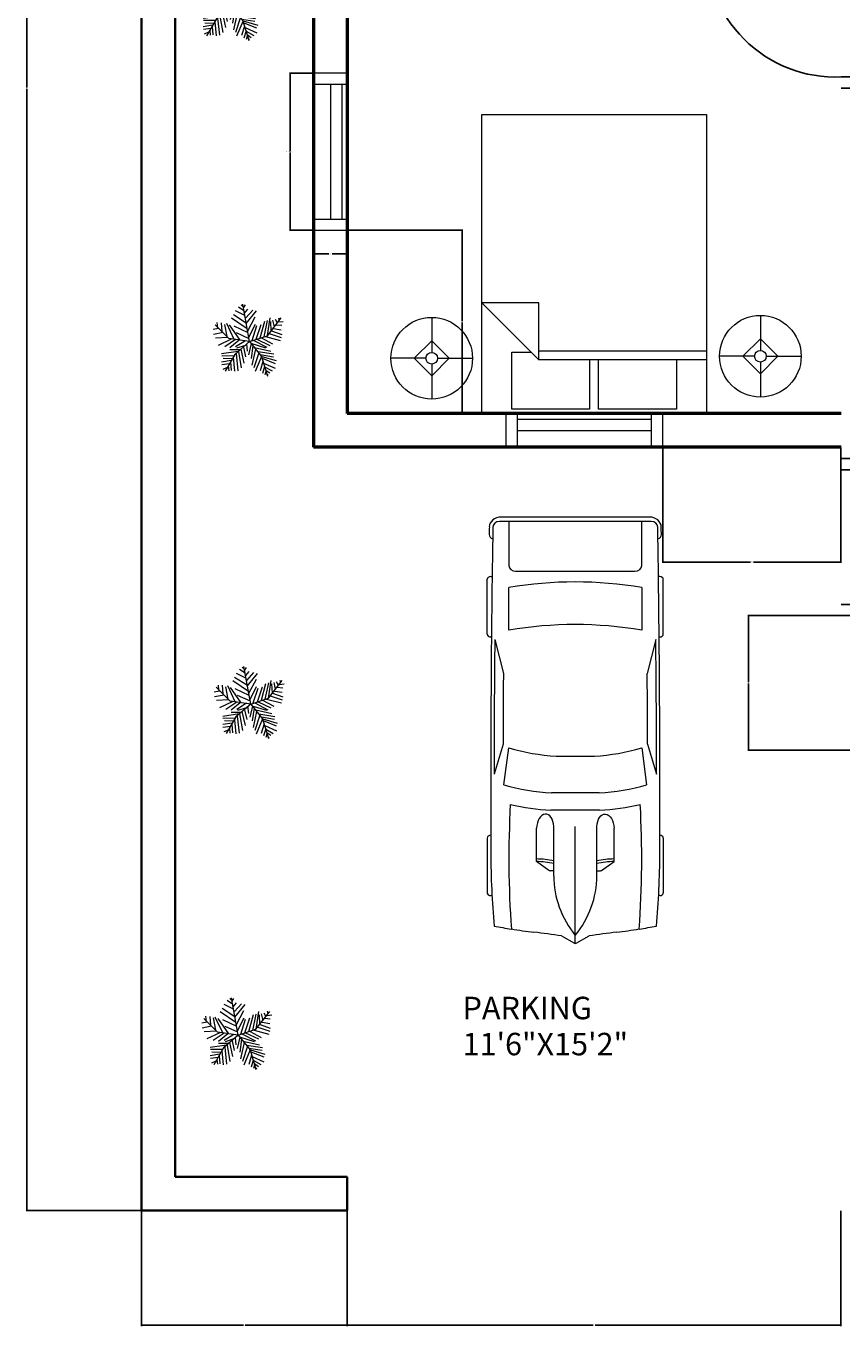
# Model space of a CAD drawing. Units: inches. Extents: x 156 to 720, y 11 to 679.
# Tile 1 of 5: x 156 to 374, y 11 to 359. Entities that reach past the tile are written whole.
import ezdxf

# ---------------------------------------------------------------- set-up
doc = ezdxf.new("R2010")
doc.units = ezdxf.units.IN
for name, color, linetype, lineweight in [('A-ANNO-DIMS', 2, 'Continuous', 18), ('A-AREA-IDEN', 7, 'Continuous', 25), ('A-DOOR', 3, 'Continuous', 25), ('A-FURN', 8, 'Continuous', 18), ('A-GLAZ', 4, 'Continuous', 18), ('A-WALL', 7, 'Continuous', 50), ('C-PKNG-VEHC', 8, 'Continuous', 13), ('C-PROP', 7, 'Continuous', 35), ('E-LITE', 2, 'Continuous', 13), ('L-PLNT', 94, 'Continuous', 13)]:
    doc.layers.add(name, color=color, linetype=linetype, lineweight=lineweight)
doc.styles.get("Standard").update_dxf_attribs({"font": 'arial.ttf'})
doc.dimstyles.get("Standard").update_dxf_attribs({"dimtxt": 0.18, "dimasz": 0.18, "dimexe": 0.18, "dimexo": 0.0625, "dimgap": 0.09, "dimtad": 0, "dimtih": 1, "dimtoh": 1, "dimdec": 4, "dimzin": 0, "dimdsep": 46, "dimtxsty": 'Standard', "dimcen": 0.09, "dimadec": 0, "dimazin": 0, "dimtfac": 1, "dimtdec": 4, "dimtofl": 0, "dimtmove": 0, "dimatfit": 3, "dimfxl": 1, "dimtolj": 1, "dimtzin": 0, "dimarcsym": 0})

# ---------------------------------------------------------------- blocks, each defined once
blk = doc.blocks.new('Bed - Queen')
for p, q in [((0, -80.00003), (0, 0)), ((0, 0), (59.99999, 0)), ((59.99999, 0), (59.99999, -80.00003)), ((7.99999, -1.2), (28.79998, -1.2)), ((7.99999, -14.4), (7.99999, -1.2)), ((28.79998, -1.2), (28.79998, -14.4)), ((31.19999, -1.2), (51.99999, -1.2)), ((31.19999, -14.4), (31.19999, -1.2)), ((51.99999, -1.2), (51.99999, -16.4)), ((0, -14.4), (44.8, -14.4)), ((44.8, -16.8), (0, -16.8)), ((59.99999, -29.6), (44.8, -14.4)), ((44.8, -14.4), (44.8, -29.6)), ((51.99999, -16.4), (46.79936, -16.4)), ((44.8, -29.6), (59.99999, -29.6)), ((59.99999, -80.00003), (0, -80.00003))]:
    blk.add_line(p, q)
blk = doc.blocks.new('Lamp - Table')
for p, q in [((0, 7), (0, 1)), ((0, 3), (-3, 0)), ((3, 0), (0, 3)), ((-1, 0), (-7, 0)), ((-3, 0), (0, -3)), ((0, -3), (3, 0)), ((1, 0), (7, 0)), ((0, -1), (0, -7))]:
    blk.add_line(p, q)
for radius in [7, 1]:
    blk.add_circle((0, 0), radius)
blk = doc.blocks.new('*U14')
for p, q in [((21.1, 37.41), (21.1, 36.83)), ((46.55, 38.89), (22.35, 38.89)), ((47.8, 37.39), (47.8, 37.41)), ((87.99, 31.87), (74.76, 35.92)), ((134.31, 35.6), (119.29, 31.78)), ((135.45, 37.07), (135.45, 37.41)), ((136.7, 38.89), (160.9, 38.89)), ((162.15, 37.41), (162.15, 36.77)), ((70.03, 31.54), (86.41, 29.35)), ((138.42, 29.35), (157.25, 29.35)), ((186.47, 29.35), (167.01, 29.35)), ((186.47, -33.5), (186.47, 33.5)), ((188.4, -32.76), (188.4, 32.76)), ((164.52, 26.39), (164.52, -26.39)), ((32.27, 11.63), (36.13, 17.17)), ((36.13, 17.17), (50.94, 17.17)), ((3.27, 6.13), (0.1, 0.41)), ((29.77, 9.51), (51.68, 9.51)), ((32.12, 9.51), (32.12, 11.15)), ((58.92, -10.77), (58.92, 10.77)), ((66.55, -10.53), (66.55, 10.53)), ((82.74, 8.5), (82.74, -8.5)), ((186.47, -10.53), (186.47, 10.53)), ((0, 0), (51.68, 0)), ((0.1, -0.41), (3.27, -6.13)), ((29.77, -9.51), (51.68, -9.51)), ((32.12, -9.51), (32.12, -11.15)), ((32.27, -11.63), (36.13, -17.17)), ((36.13, -17.17), (50.94, -17.17)), ((86.41, -29.35), (70.03, -31.54)), ((87.99, -31.87), (74.76, -35.92)), ((134.31, -35.6), (119.29, -31.78)), ((157.25, -29.35), (138.42, -29.35)), ((167.01, -29.35), (186.47, -29.35)), ((21.1, -37.41), (21.1, -36.83)), ((46.55, -38.89), (22.35, -38.89)), ((47.8, -37.39), (47.8, -37.41)), ((135.45, -37.07), (135.45, -37.41)), ((136.7, -38.89), (160.9, -38.89)), ((162.15, -37.41), (162.15, -36.77))]:
    blk.add_line(p, q)
for centre, major_axis, ratio, start_param, end_param in [((266.03, -27.52), (0, 313.31), 0.842304, 1.367076, 1.39176), ((41.19, -490.86), (0, 528.23), 0.842304, 0.00281, 0.075598), ((22.35, 37.41), (0, -1.48), 0.842304, 3.141593, 4.712389), ((64.48, -10555.62), (0, 10593.03), 0.842304, -0.013397, 0.002797), ((46.55, 37.41), (0, 1.48), 0.842304, -1.570796, 0), ((64.48, -10555.62), (0, -10591.55), 0.842304, 3.133765, 3.140441), ((136.7, 37.41), (0, -1.48), 0.842304, 3.141593, 4.712389), ((160.9, 37.41), (0, 1.48), 0.842304, -1.570796, 0), ((180.63, 35.84), (0, 2.22), 0.842304, -0.013017, 1.249894), ((64.48, -10556.36), (0, 10595.31), 0.842304, -0.013397, -0.013017), ((183.98, 33.5), (0, -2.96), 0.842304, 1.570796, 3.128196), ((183.98, 32.76), (0, -5.25), 0.842304, 1.570796, 3.128196), ((37.47, -593.96), (0, -623.33), 0.842304, 3.096046, 3.200911), ((135.29, 5.39), (0, 81.77), 0.842304, 1.245306, 1.50788), ((149.6, 2.8), (0, -79.58), 0.842304, 4.372215, 4.640744), ((95.79, -3666.35), (0, -3698.24), 0.842304, 3.134049, 3.144098), ((17.08, 0), (0, 147.02), 0.842304, 4.511394, 4.913384), ((35.91, 0), (0, 147.02), 0.842304, 4.511394, 4.913384), ((167.01, 26.39), (0, 2.96), 0.842304, 0, 1.570796), ((259.18, -27.52), (0, -305.3), 0.842304, 4.528606, 4.561838), ((134.4, 5.39), (0, -89.78), 0.842304, 4.449482, 4.652344), ((-204.49, 52.4), (0, -250.96), 0.842304, 1.385369, 1.434372), ((32.75, 11.15), (0, 0.74), 0.842304, 0.879714, 1.570796), ((13.04, 17.01), (0, 27.42), 0.842304, 4.435146, 4.718221), ((14.2, 17.01), (0, 27.42), 0.842304, 4.435146, 4.718221), ((50.79, 13.34), (6.34, -0.36), 0.603834, -1.395552, 1.581315), ((29.77, -46.66), (0, 56.17), 0.842304, 0, 0.590319), ((0.62, 0), (0, -0.74), 0.842304, 4.131459, 5.293319), ((29.77, 46.66), (0, 56.17), 0.842304, 2.551274, 3.141593), ((-204.49, -52.4), (0, 250.96), 0.842304, -1.434372, -1.385369), ((32.75, -11.15), (0, -0.74), 0.842304, 4.712389, 5.403472), ((13.04, -17.01), (0, -27.42), 0.842304, 1.564964, 1.848039), ((14.2, -17.01), (0, -27.42), 0.842304, 1.564964, 1.848039), ((134.4, -5.39), (0, -89.78), 0.842304, -1.510751, -1.307889), ((135.29, -5.39), (0, -81.77), 0.842304, -1.50788, -1.245306), ((149.6, -2.8), (0, -79.58), 0.842304, -1.499151, -1.230623), ((259.18, 27.52), (0, 305.3), 0.842304, 1.721348, 1.754579), ((266.03, 27.52), (0, 313.31), 0.842304, 1.749832, 1.774517), ((37.47, 593.96), (0, -623.33), 0.842304, -0.059319, 0.045547), ((167.01, -26.39), (0, -2.96), 0.842304, 4.712389, 6.283185), ((95.79, 3666.35), (0, -3698.24), 0.842304, -0.002505, 0.007544), ((183.98, -33.5), (0, 2.96), 0.842304, 3.15499, 4.712389), ((183.98, -32.76), (0, -5.25), 0.842304, 0.013397, 1.570796), ((41.19, 490.86), (0, -528.23), 0.842304, -0.075598, -0.00281), ((22.35, -37.41), (0, 1.48), 0.842304, 1.570796, 3.141593), ((64.48, 10555.62), (0, 10593.03), 0.842304, 3.138796, 3.15499), ((46.55, -37.41), (0, -1.48), 0.842304, 0, 1.570796), ((64.48, 10555.62), (0, -10591.55), 0.842304, 0.001152, 0.007828), ((136.7, -37.41), (0, -1.48), 0.842304, -1.570796, 0), ((160.9, -37.41), (0, 1.48), 0.842304, 3.141593, 4.712389), ((180.63, -35.84), (0, -2.22), 0.842304, -1.249894, 0.013017), ((64.48, 10556.36), (0, 10595.31), 0.842304, 3.15461, 3.15499)]:
    blk.add_ellipse(centre, major_axis=major_axis, ratio=ratio, start_param=start_param, end_param=end_param)
at = {"extrusion": (0, 0, -1)}
blk.add_ellipse((50.79, -13.34), major_axis=(6.34, 0.36), ratio=0.603834, start_param=-1.395552, end_param=1.581315, dxfattribs=at)
blk = doc.blocks.new('*U13')
for p, q in [((-5.114, 28.097), (-24.676, 40.636)), ((-7.288, 39.707), (-21.778, 46.673)), ((-8.737, 47.138), (-17.069, 52.711)), ((-10.186, 53.64), (-13.084, 55.962)), ((0, 0), (-10.5, 57)), ((-9.099, 51.782), (-6.563, 55.962)), ((-7.65, 43.423), (-2.578, 49.46)), ((-5.839, 35.992), (4.667, 48.067)), ((-5.114, 27.632), (10.463, 46.673)), ((-31.5, 4.5), (-52.5, 25.5)), ((-48.585, 21.131), (-49.309, 29.026)), ((-43.513, 28.561), (-42.427, 15.558)), ((-38.442, 26.239), (-34.819, 7.663)), ((-35.544, 28.097), (-24.314, 3.947)), ((-14.533, 2.09), (-30.834, 25.31)), ((-3.665, 19.273), (-27.574, 35.527)), ((-24.314, 23.917), (-2.941, 13.7)), ((-2.941, 16.486), (8.652, 37.85)), ((-1.129, 6.734), (9.014, 26.704)), ((3.942, 1.625), (11.187, 24.381)), ((10.101, 3.483), (17.708, 26.239)), ((16.259, 5.805), (23.142, 31.348)), ((22.055, 7.198), (27.489, 32.277)), ((27, 9), (48, 36)), ((27.127, 9.056), (31.112, 35.992)), ((31.836, 30.883), (32.561, 16.486)), ((35.096, 32.741), (37.27, 22.524)), ((38.719, 34.134), (41.979, 28.561)), ((40.53, 25.775), (48.862, 24.846)), ((43.791, 29.954), (51.036, 30.883)), ((44.153, 36.456), (45.239, 32.741)), ((-47.498, 19.737), (-55.83, 18.344)), ((-40.615, 13.7), (-55.105, 10.913)), ((-33.37, 6.269), (-52.207, 5.34)), ((-28.299, 3.483), (-47.86, -5.805)), ((-21.416, 3.018), (-38.079, -8.128)), ((0, 0), (-31.5, 4.5)), ((-15.982, 2.09), (-30.11, -9.521)), ((0, 0), (-22.5, -19.5)), ((-6.563, 1.161), (-21.416, -8.128)), ((-20.691, 13.7), (-1.129, 4.876)), ((0, 0), (27, 9)), ((0, 0), (18, -22.5)), ((6.478, 1.625), (26.04, -8.592)), ((11.187, 3.483), (30.749, -5.805)), ((18.07, 5.805), (35.096, -3.483)), ((24.229, 7.663), (46.688, 1.625)), ((29.662, 12.307), (48.137, 6.269)), ((33.285, 16.486), (48.862, 10.913)), ((36.183, 19.737), (48.137, 17.88)), ((-17.431, -15.094), (-42.789, -18.809)), ((-22.5, -19.5), (-37.5, -45)), ((-15.257, -12.772), (-30.11, -12.772)), ((-20.691, -18.345), (-17.793, -44.352)), ((-6.563, -5.805), (-19.967, -9.985)), ((-17.069, -15.094), (-12.721, -40.172)), ((-13.446, -11.378), (-8.737, -32.741)), ((-9.461, -8.592), (-6.201, -23.453)), ((-4.752, -3.483), (-3.665, -14.629)), ((2.493, -3.019), (-1.491, -20.202)), ((1.769, -2.555), (24.229, -9.521)), ((5.029, -6.27), (2.131, -25.775)), ((9.014, -11.378), (3.58, -35.992)), ((14.085, -16.951), (6.478, -40.172)), ((7.565, -9.056), (32.198, -14.629)), ((12.274, -15.094), (36.907, -18.809)), ((16.259, -19.738), (36.183, -22.989)), ((-28.299, -29.026), (-42.789, -31.348)), ((-24.314, -21.596), (-42.427, -22.06)), ((-30.834, -34.135), (-42.427, -35.528)), ((-26.849, -26.24), (-40.253, -25.775)), ((-32.646, -36.921), (-31.921, -44.352)), ((-29.023, -30.884), (-27.936, -43.887)), ((-25.038, -23.918), (-22.865, -45.281)), ((18.07, -22.524), (8.289, -45.745)), ((20.244, -30.419), (15.897, -44.816)), ((18, -22.5), (27, -52.5)), ((18.433, -22.524), (40.53, -29.026)), ((19.157, -25.311), (38.719, -33.206)), ((22.78, -37.85), (19.519, -48.532)), ((21.331, -32.741), (39.081, -40.636)), ((22.78, -38.314), (34.372, -44.816)), ((-34.457, -39.708), (-40.978, -42.494)), ((24.591, -45.745), (23.142, -50.854)), ((24.591, -43.423), (30.749, -47.603)), ((26.764, -49.925), (28.213, -50.854))]:
    blk.add_line(p, q)
blk = doc.blocks.new('DOOR-SWING-36IN')
for p, q in [((0, 6), (0, 0)), ((3, 6), (3, 0)), ((39, 6), (39, 0)), ((42, 6), (42, 0))]:
    blk.add_line(p, q)
blk.add_lwpolyline([(39, 6), (36, 6), (36, 42), (39, 42)], close=True)
blk.add_arc((37.5, 7.5), 34.53, 87.5104, 182.4896)
blk = doc.blocks.new('WIN-36IN-WALL9')
for p, q in [((0, 9), (0, 0)), ((39, 9), (3, 9)), ((3, 9), (3, 0)), ((3, 7.5), (39, 7.5)), ((39, 0), (39, 9)), ((42, 0), (42, 9)), ((3, 4.5), (39, 4.5)), ((3, 0), (39, 0))]:
    blk.add_line(p, q)
blk = doc.blocks.new('*D29')
at = {"layer": 'A-ANNO-DIMS', "color": 0, "lineweight": -2, "transparency": 16777216}
for p, q in [((232.66, 346.15), (226.24, 346.15)), ((226.42, 345.97), (226.42, 325.33)), ((226.42, 304.33), (226.42, 324.97)), ((232.66, 304.15), (226.24, 304.15))]:
    blk.add_line(p, q, dxfattribs=at)
at = {"layer": 'A-ANNO-DIMS', "color": 0, "transparency": 16777216}
for points in [[(226.39, 345.97), (226.45, 345.97), (226.42, 346.15)], [(226.39, 304.33), (226.45, 304.33), (226.42, 304.15)]]:
    blk.add_solid(points, dxfattribs=at)
at = {"layer": 'Defpoints', "color": 0, "transparency": 16777216}
for p in [(232.72, 346.15), (226.42, 304.15), (232.72, 304.15)]:
    blk.add_point(p, dxfattribs=at)
at = {"layer": 'A-ANNO-DIMS', "color": 0, "transparency": 16777216, "insert": (226.42, 325.15), "char_height": 0.18, "attachment_point": 5}
blk.add_mtext('\\A1;WINDOW A 42 TYP.', dxfattribs=at)
blk = doc.blocks.new('*D30')
at = {"layer": 'A-ANNO-DIMS', "color": 0, "lineweight": -2, "transparency": 16777216}
for p, q in [((232.72, 304.09), (232.72, 297.67)), ((241.72, 304.09), (241.72, 297.67)), ((232.9, 297.85), (236.77, 297.85)), ((241.54, 297.85), (237.68, 297.85))]:
    blk.add_line(p, q, dxfattribs=at)
at = {"layer": 'A-ANNO-DIMS', "color": 0, "transparency": 16777216}
for points in [[(232.9, 297.88), (232.9, 297.82), (232.72, 297.85)], [(241.54, 297.88), (241.54, 297.82), (241.72, 297.85)]]:
    blk.add_solid(points, dxfattribs=at)
at = {"layer": 'Defpoints', "color": 0, "transparency": 16777216}
for p in [(232.72, 304.15), (241.72, 304.15), (241.72, 297.85)]:
    blk.add_point(p, dxfattribs=at)
at = {"layer": 'A-ANNO-DIMS', "color": 0, "transparency": 16777216, "insert": (237.22, 297.85), "char_height": 0.18, "attachment_point": 5}
blk.add_mtext('\\A1;9 TYP.', dxfattribs=at)
blk = doc.blocks.new('*D50')
at = {"layer": 'A-ANNO-DIMS', "color": 0, "lineweight": -2, "transparency": 16777216}
for p, q in [((186.66, 642.15), (155.84, 642.15)), ((156.02, 641.97), (156.02, 342.33)), ((156.02, 42.33), (156.02, 341.97)), ((186.66, 42.15), (155.84, 42.15))]:
    blk.add_line(p, q, dxfattribs=at)
at = {"layer": 'A-ANNO-DIMS', "color": 0, "transparency": 16777216}
for points in [[(155.99, 641.97), (156.05, 641.97), (156.02, 642.15)], [(155.99, 42.33), (156.05, 42.33), (156.02, 42.15)]]:
    blk.add_solid(points, dxfattribs=at)
at = {"layer": 'Defpoints', "color": 0, "transparency": 16777216}
for p in [(156.02, 642.15), (186.72, 642.15), (186.72, 42.15)]:
    blk.add_point(p, dxfattribs=at)
at = {"layer": 'A-ANNO-DIMS', "color": 0, "transparency": 16777216, "insert": (156.02, 342.15), "char_height": 0.18, "attachment_point": 5}
blk.add_mtext('\\A1;600', dxfattribs=at)
blk = doc.blocks.new('*D51')
at = {"layer": 'A-ANNO-DIMS', "color": 0, "lineweight": -2, "transparency": 16777216}
for p, q in [((186.72, 42.09), (186.72, 11.27)), ((241.72, 42.09), (241.72, 11.27)), ((186.9, 11.45), (214, 11.45)), ((241.54, 11.45), (214.44, 11.45))]:
    blk.add_line(p, q, dxfattribs=at)
at = {"layer": 'A-ANNO-DIMS', "color": 0, "transparency": 16777216}
for points in [[(186.9, 11.48), (186.9, 11.42), (186.72, 11.45)], [(241.54, 11.48), (241.54, 11.42), (241.72, 11.45)]]:
    blk.add_solid(points, dxfattribs=at)
at = {"layer": 'Defpoints', "color": 0, "transparency": 16777216}
for p in [(186.72, 42.15), (241.72, 42.15), (241.72, 11.45)]:
    blk.add_point(p, dxfattribs=at)
at = {"layer": 'A-ANNO-DIMS', "color": 0, "transparency": 16777216, "insert": (214.22, 11.45), "char_height": 0.18, "attachment_point": 5}
blk.add_mtext('\\A1;55', dxfattribs=at)
blk = doc.blocks.new('*D52')
at = {"layer": 'A-ANNO-DIMS', "color": 0, "lineweight": -2, "transparency": 16777216}
for p, q in [((241.72, 42.09), (241.72, 11.27)), ((373.72, 42.09), (373.72, 11.27)), ((241.9, 11.45), (307.44, 11.45)), ((373.54, 11.45), (308, 11.45))]:
    blk.add_line(p, q, dxfattribs=at)
at = {"layer": 'A-ANNO-DIMS', "color": 0, "transparency": 16777216}
for points in [[(241.9, 11.48), (241.9, 11.42), (241.72, 11.45)], [(373.54, 11.48), (373.54, 11.42), (373.72, 11.45)]]:
    blk.add_solid(points, dxfattribs=at)
at = {"layer": 'Defpoints', "color": 0, "transparency": 16777216}
for p in [(241.72, 42.15), (373.72, 42.15), (373.72, 11.45)]:
    blk.add_point(p, dxfattribs=at)
at = {"layer": 'A-ANNO-DIMS', "color": 0, "transparency": 16777216, "insert": (307.72, 11.45), "char_height": 0.18, "attachment_point": 5}
blk.add_mtext('\\A1;132', dxfattribs=at)
blk = doc.blocks.new('*D68')
at = {"layer": 'A-ANNO-DIMS', "color": 0, "lineweight": -2, "transparency": 16777216}
for p, q in [((379.66, 201.15), (348.84, 201.15)), ((349.02, 200.97), (349.02, 183.33)), ((349.02, 165.33), (349.02, 182.97)), ((379.66, 165.15), (348.84, 165.15))]:
    blk.add_line(p, q, dxfattribs=at)
at = {"layer": 'A-ANNO-DIMS', "color": 0, "transparency": 16777216}
for points in [[(348.99, 200.97), (349.05, 200.97), (349.02, 201.15)], [(348.99, 165.33), (349.05, 165.33), (349.02, 165.15)]]:
    blk.add_solid(points, dxfattribs=at)
at = {"layer": 'Defpoints', "color": 0, "transparency": 16777216}
for p in [(349.02, 201.15), (379.72, 201.15), (379.72, 165.15)]:
    blk.add_point(p, dxfattribs=at)
at = {"layer": 'A-ANNO-DIMS', "color": 0, "transparency": 16777216, "insert": (349.02, 183.15), "char_height": 0.18, "attachment_point": 5}
blk.add_mtext('\\A1;36', dxfattribs=at)
blk = doc.blocks.new('*D73')
at = {"layer": 'A-ANNO-DIMS', "color": 0, "lineweight": -2, "transparency": 16777216}
for p, q in [((241.79, 304.15), (272.6, 304.15)), ((272.42, 303.97), (272.42, 279.83)), ((272.42, 255.33), (272.42, 279.47)), ((241.79, 255.15), (272.6, 255.15))]:
    blk.add_line(p, q, dxfattribs=at)
at = {"layer": 'A-ANNO-DIMS', "color": 0, "transparency": 16777216}
for points in [[(272.39, 303.97), (272.45, 303.97), (272.42, 304.15)], [(272.39, 255.33), (272.45, 255.33), (272.42, 255.15)]]:
    blk.add_solid(points, dxfattribs=at)
at = {"layer": 'Defpoints', "color": 0, "transparency": 16777216}
for p in [(241.72, 304.15), (241.72, 255.15), (272.42, 255.15)]:
    blk.add_point(p, dxfattribs=at)
at = {"layer": 'A-ANNO-DIMS', "color": 0, "transparency": 16777216, "insert": (272.42, 279.65), "char_height": 0.18, "attachment_point": 5}
blk.add_mtext('\\A1;49', dxfattribs=at)
blk = doc.blocks.new('*D74')
at = {"layer": 'A-ANNO-DIMS', "color": 0, "lineweight": -2, "transparency": 16777216}
for p, q in [((326.1, 246.09), (326.1, 215.27)), ((373.72, 246.09), (373.72, 215.27)), ((326.28, 215.45), (349.52, 215.45)), ((373.54, 215.45), (350.31, 215.45))]:
    blk.add_line(p, q, dxfattribs=at)
at = {"layer": 'A-ANNO-DIMS', "color": 0, "transparency": 16777216}
for points in [[(326.28, 215.48), (326.28, 215.42), (326.1, 215.45)], [(373.54, 215.48), (373.54, 215.42), (373.72, 215.45)]]:
    blk.add_solid(points, dxfattribs=at)
at = {"layer": 'Defpoints', "color": 0, "transparency": 16777216}
for p in [(326.1, 246.15), (373.72, 246.15), (326.1, 215.45)]:
    blk.add_point(p, dxfattribs=at)
at = {"layer": 'A-ANNO-DIMS', "color": 0, "transparency": 16777216, "insert": (349.91, 215.45), "char_height": 0.18, "attachment_point": 5}
blk.add_mtext('\\A1;47.62', dxfattribs=at)

msp = doc.modelspace()

# ---------------------------------------------------------------- linework, layer by layer
at = {"layer": 'A-WALL'}
for p, q in [((232.7236, 633.1514), (232.7236, 246.1514)), ((241.7236, 387.1514), (241.7236, 255.1514)), ((373.7236, 255.1514), (241.7236, 255.1514)), ((373.7236, 246.1514), (232.7236, 246.1514))]:
    msp.add_line(p, q, dxfattribs=at)
at = {"layer": 'C-PROP'}
for p, q in [((186.7236, 642.1514), (186.7236, 51.1514)), ((195.7236, 633.1514), (195.7236, 51.1514)), ((186.7236, 51.1514), (186.7236, 42.1514)), ((195.7236, 51.1514), (241.7236, 51.1514)), ((241.7236, 51.1514), (241.7236, 42.1514)), ((189.7236, 42.1514), (186.7236, 42.1514)), ((189.7236, 42.1514), (241.7236, 42.1514))]:
    msp.add_line(p, q, dxfattribs=at)

# ---------------------------------------------------------------- block references
at = {"layer": 'A-DOOR', "rotation": 89.99999999999989}
msp.add_blockref('DOOR-SWING-36IN', (379.724, 342.1518), dxfattribs=at)
at = {"layer": 'A-DOOR', "extrusion": (0, 0, -1), "zscale": -1, "rotation": 89.99999999999999}
msp.add_blockref('DOOR-SWING-36IN', (-373.7232, 201.1518), dxfattribs=at)
at = {"layer": 'A-FURN', "rotation": 180}
msp.add_blockref('Bed - Queen', (337.7236, 255.1514), dxfattribs=at)
at = {"layer": 'A-GLAZ', "rotation": 270.0000000000002}
msp.add_blockref('WIN-36IN-WALL9', (232.7232, 346.151), dxfattribs=at)
at = {"layer": 'A-GLAZ'}
msp.add_blockref('WIN-36IN-WALL9', (284.1, 246.151), dxfattribs=at)
at = {"layer": 'C-PKNG-VEHC', "xscale": 0.6047966740307916, "yscale": 0.6047966740307916, "zscale": 0.6047966740307916, "rotation": 90}
msp.add_blockref('*U14', (302.6843, 113.547), dxfattribs=at)
at = {"layer": 'E-LITE', "xscale": 1.558829175044203, "yscale": 1.558829175044203, "zscale": 1.558829175044203}
for p in [(264.292, 269.9596), (352.1694, 270.4966)]:
    msp.add_blockref('Lamp - Table', p, dxfattribs=at)
at = {"layer": 'L-PLNT', "xscale": 0.175286236255467, "yscale": 0.175286236255467, "zscale": 0.175286236255467}
for p in [(210.6733, 364.0639), (215.6146, 274.4057), (215.9103, 177.5226), (212.5798, 89.0055)]:
    msp.add_blockref('*U13', p, dxfattribs=at)

# ---------------------------------------------------------------- texts
at = {"layer": 'A-AREA-IDEN'}
for s, p in [('PARKING', (272.5366, 93.2714)), ('11\'6"X15\'2"', (272.5366, 83.6329))]:
    msp.add_text(s, height=6, dxfattribs=at).set_placement(p)

# ---------------------------------------------------------------- dimensions: what is measured, and where the dimension line sits
at = {"layer": 'A-ANNO-DIMS'}
for base, p1, p2, angle, override, picture, middle in [((156.0236, 642.1514), (186.7236, 42.1514), (186.7236, 642.1514), 90, {"dimdec": 0, "dimlfac": 1, "dimrnd": 0, "dimzin": 0, "dimdsep": 46, "dimlunit": 2}, '*D50', (156.0236, 342.1514)), ((272.4236, 255.1514), (241.7236, 304.1508), (241.7236, 255.1514), 270, {"dimdec": 0, "dimlfac": 1, "dimrnd": 0, "dimzin": 0, "dimdsep": 46, "dimlunit": 2}, '*D73', (272.4236, 279.6511)), ((326.1002, 215.4514), (373.7236, 246.1514), (326.1002, 246.1514), 180, {"dimdec": 2, "dimlfac": 1, "dimrnd": 0, "dimzin": 0, "dimdsep": 46, "dimlunit": 2}, '*D74', (349.9119, 215.4514)), ((349.0236, 201.1514), (379.7236, 165.1514), (379.7236, 201.1514), 90, {"dimdec": 0, "dimlfac": 1, "dimrnd": 0, "dimzin": 0, "dimdsep": 46, "dimlunit": 2}, '*D68', (349.0236, 183.1514))]:
    dim = msp.add_linear_dim(base=base, p1=p1, p2=p2, angle=angle, dimstyle='Standard', override=override, dxfattribs=at)
    dim.commit()
    dim.dimension.update_dxf_attribs({"geometry": picture, "text_midpoint": middle})
for base, p1, p2, angle, text, picture, middle in [((226.4236, 304.1508), (232.7236, 346.1508), (232.7236, 304.1508), 270, 'WINDOW A <> TYP.', '*D29', (226.4236, 325.1508)), ((241.7236, 297.8508), (232.7236, 304.1508), (241.7236, 304.1508), 0, '<> TYP.', '*D30', (237.2236, 297.8508))]:
    dim = msp.add_linear_dim(base=base, p1=p1, p2=p2, angle=angle, text=text, dimstyle='Standard', override={"dimdec": 0, "dimlfac": 1, "dimrnd": 0, "dimzin": 0, "dimdsep": 46, "dimlunit": 2}, dxfattribs=at)
    dim.commit()
    dim.dimension.update_dxf_attribs({"geometry": picture, "text_midpoint": middle})
for base, p1, p2, picture, middle in [((241.7236, 11.4514), (186.7236, 42.1514), (241.7236, 42.1514), '*D51', (214.2236, 11.4514)), ((373.7236, 11.4514), (241.7236, 42.1514), (373.7236, 42.1514), '*D52', (307.7236, 11.4514))]:
    dim = msp.add_linear_dim(base=base, p1=p1, p2=p2, dimstyle='Standard', override={"dimdec": 0, "dimlfac": 1, "dimrnd": 0, "dimzin": 0, "dimdsep": 46, "dimlunit": 2}, dxfattribs=at)
    dim.commit()
    dim.dimension.update_dxf_attribs({"geometry": picture, "text_midpoint": middle})

doc.saveas('drawing.dxf')
